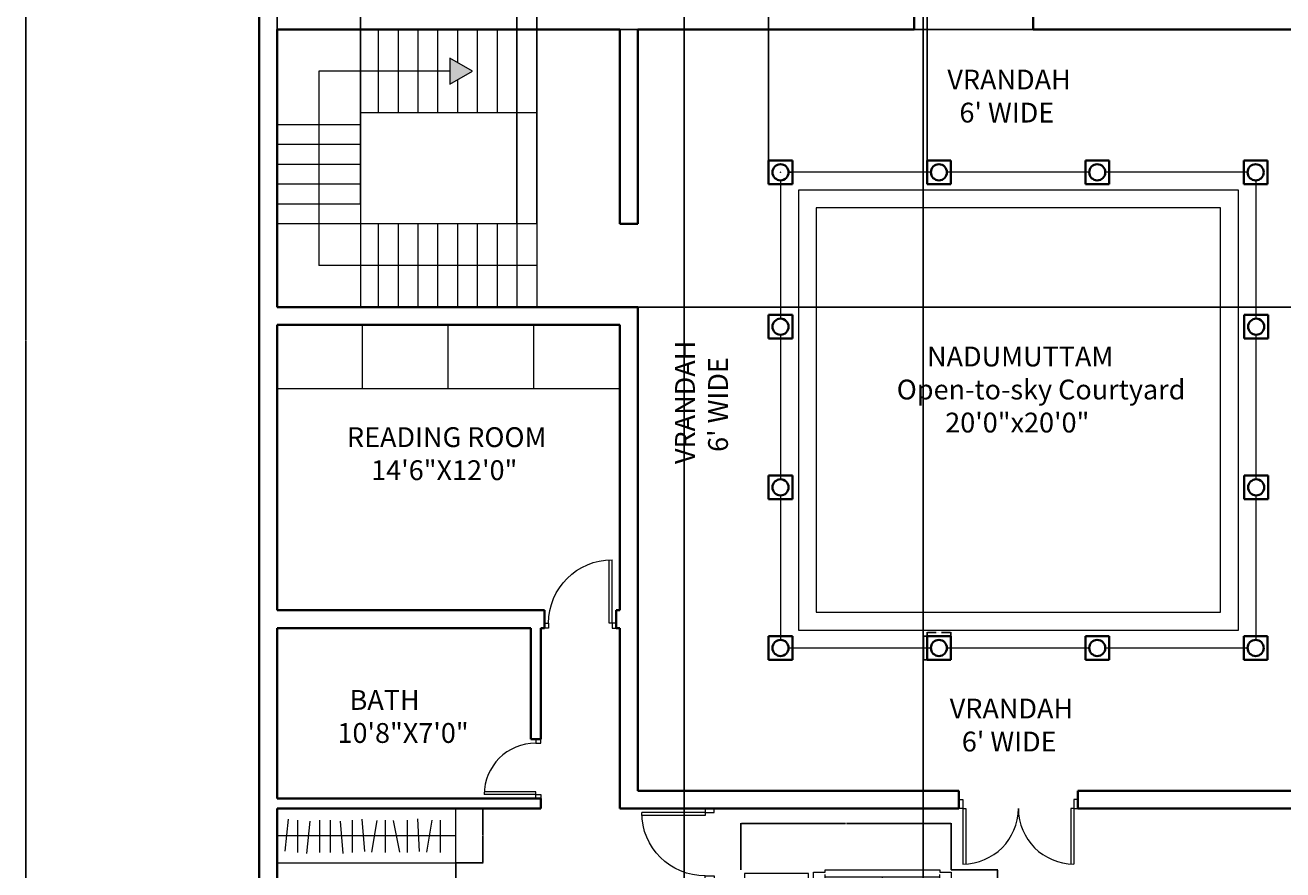
# Model space of a CAD drawing. Units: inches. Extents: x 4602 to 5612, y 5125 to 6591.
# Tile 2 of 6: x 4602 to 5237, y 5551 to 5977. Entities that reach past the tile are written whole.
import ezdxf

# ---------------------------------------------------------------- set-up
doc = ezdxf.new("R2010")
doc.units = ezdxf.units.IN
for name, color, linetype, lineweight in [('A-ANNO-DIMS', 2, 'Continuous', 18), ('A-ANNO-PATT', 7, 'Continuous', 18), ('A-ANNO-SYMB', 7, 'Continuous', 18), ('A-AREA-IDEN', 7, 'Continuous', 18), ('A-COLS', 7, 'Continuous', 35), ('A-DOOR', 4, 'Continuous', 18), ('A-FLOR-CASE', 9, 'Continuous', 18), ('A-FLOR-EDGE', 7, 'Continuous', 18), ('A-FLOR-STRS', 7, 'Continuous', 18), ('A-FURN', 8, 'Continuous', 13), ('A-WALL', 7, 'Continuous', 35)]:
    doc.layers.add(name, color=color, linetype=linetype, lineweight=lineweight)
doc.styles.get("Standard").update_dxf_attribs({"font": 'arial.ttf'})
doc.dimstyles.get("Standard").update_dxf_attribs({"dimtxt": 0.18, "dimasz": 0.18, "dimexe": 0.18, "dimexo": 0.0625, "dimgap": 0.09, "dimtad": 0, "dimtih": 1, "dimtoh": 1, "dimdec": 4, "dimzin": 0, "dimdsep": 46, "dimtxsty": 'Standard', "dimcen": 0.09, "dimadec": 0, "dimazin": 0, "dimtfac": 1, "dimtdec": 4, "dimtofl": 0, "dimtmove": 0, "dimatfit": 3, "dimfxl": 1, "dimtolj": 1, "dimtzin": 0, "dimarcsym": 0})

# ---------------------------------------------------------------- blocks, each defined once
blk = doc.blocks.new('A$C1C981678')
for p, q in [((0, 1425), (0, 2066)), ((0, 2066), (591, 2066)), ((55, 1480), (55, 2011)), ((55, 2011), (536, 2011)), ((536, 2011), (536, 1480)), ((591, 2066), (591, 1425)), ((643, 1571), (643, 2074)), ((643, 2074), (757, 2074)), ((757, 2097), (2312, 2097)), ((757, 2074), (757, 2097)), ((757, 1571), (757, 2074)), ((757, 2028), (2312, 2028)), ((1283, 1342), (1283, 2028)), ((1786, 1342), (1786, 2028)), ((2312, 2097), (2312, 2074)), ((2312, 2074), (2426, 2074)), ((2312, 1571), (2312, 2074)), ((2426, 2074), (2426, 1571)), ((2463, 2062), (2463, 1422)), ((3055, 2062), (2463, 2062)), ((3055, 1422), (3055, 2062)), ((2519, 2007), (2519, 1477)), ((3000, 2007), (2519, 2007)), ((3000, 1477), (3000, 2007)), ((287, 1770), (287, 1869)), ((2312, 1868), (757, 1868)), ((2312, 1822), (757, 1822)), ((2312, 1777), (757, 1777)), ((2773, 1759), (2773, 1859)), ((264, 1747), (165, 1747)), ((287, 1724), (287, 1625)), ((310, 1747), (409, 1747)), ((2750, 1737), (2651, 1737)), ((2773, 1714), (2773, 1615)), ((2796, 1737), (2895, 1737)), ((689, 1548), (643, 1571)), ((689, 1479), (689, 1548)), ((689, 1548), (734, 1548)), ((734, 1548), (757, 1571)), ((757, 1479), (757, 1571)), ((2335, 1548), (2312, 1571)), ((2312, 1479), (2312, 1571)), ((2380, 1548), (2335, 1548)), ((2426, 1571), (2380, 1548)), ((2380, 1548), (2380, 1479)), ((591, 1425), (0, 1425)), ((536, 1480), (55, 1480)), ((757, 1479), (689, 1479)), ((757, 1342), (757, 1479)), ((2380, 1479), (2312, 1479)), ((2312, 1479), (2312, 1342)), ((2463, 1422), (3055, 1422)), ((2519, 1477), (3000, 1477)), ((17, 1295), (17, 746)), ((40, 1295), (17, 1295)), ((634, 1364), (40, 1364)), ((40, 1364), (40, 1295)), ((108, 1295), (40, 1295)), ((345, 1295), (108, 1295)), ((108, 1295), (108, 746)), ((245, 746), (245, 1295)), ((295, 746), (295, 1295)), ((345, 746), (345, 1295)), ((345, 1295), (634, 1295)), ((634, 1295), (634, 1364)), ((680, 1295), (634, 1295)), ((680, 746), (680, 1295)), ((2312, 1342), (757, 1342)), ((2337, 114), (2337, 1257)), ((2337, 1257), (2475, 1257)), ((2475, 1326), (2543, 1326)), ((2475, 1257), (2475, 1326)), ((2475, 1257), (2566, 1257)), ((2543, 1326), (2566, 1372)), ((2543, 1326), (2543, 1280)), ((2543, 1280), (2566, 1257)), ((2566, 1372), (3069, 1372)), ((2566, 1257), (3046, 1257)), ((2772, 114), (2772, 1257)), ((2817, 114), (2817, 1257)), ((2863, 114), (2863, 1257)), ((3023, 1257), (3023, 114)), ((3069, 1372), (3069, 1257)), ((3069, 1257), (3092, 1257)), ((3092, 1257), (3092, 114)), ((1995, 1003), (1232, 1003)), ((1232, 1003), (1232, 659)), ((1960, 969), (1266, 969)), ((1266, 969), (1266, 694)), ((1960, 694), (1960, 969)), ((1995, 659), (1995, 1003)), ((17, 746), (40, 746)), ((40, 746), (40, 678)), ((108, 746), (40, 746)), ((40, 678), (634, 678)), ((108, 746), (345, 746)), ((634, 746), (345, 746)), ((634, 746), (680, 746)), ((634, 678), (634, 746)), ((1232, 659), (1995, 659)), ((1266, 694), (1960, 694)), ((2337, 686), (3023, 686)), ((2475, 114), (2337, 114)), ((2475, 46), (2475, 114)), ((2475, 114), (2566, 114)), ((2543, 46), (2475, 46)), ((2543, 91), (2566, 114)), ((2543, 46), (2543, 91)), ((2566, 0), (2543, 46)), ((2566, 114), (3046, 114)), ((3069, 0), (2566, 0)), ((3092, 114), (3069, 114)), ((3069, 114), (3069, 0))]:
    blk.add_line(p, q)
for radius in [122, 22.9]:
    blk.add_circle((2773, 1737), radius)
for major_axis in [(-86.2, 86.2), (16.2, 16.2)]:
    blk.add_ellipse((287, 1747), major_axis=major_axis, ratio=1)
blk = doc.blocks.new('DOOR-PAIR-60IN')
for p, q in [((2, 4.5), (2, 32.5)), ((3.5, 4.5), (3.5, 32.46)), ((56.5, 4.5), (56.5, 32.46)), ((58, 4.5), (58, 32.5)), ((2, 4.5), (0, 4.5)), ((2, 0), (2, 4.5)), ((2, 4.5), (3.5, 4.5)), ((58, 4.5), (56.5, 4.5)), ((58, 0), (58, 4.5)), ((58, 4.5), (60, 4.5)), ((0, 0), (2, 0)), ((60, 0), (58, 0))]:
    blk.add_line(p, q)
for centre, start, end in [((2, 4.5), 0, 90), ((58, 4.5), 90, 180)]:
    blk.add_arc(centre, 28, start, end)
blk = doc.blocks.new('DOOR-36IN-DEEP-JAMB')
for p, q in [((2, 4.5), (2, 36.5)), ((3.5, 4.5), (3.5, 36.46)), ((0, 4.5), (2, 4.5)), ((2, 4.5), (2, 0)), ((2, 4.5), (3.5, 4.5)), ((36, 4.5), (34, 4.5)), ((34, 4.5), (34, 0)), ((2, 0), (0, 0)), ((34, 0), (36, 0))]:
    blk.add_line(p, q)
blk.add_arc((2, 4.5), 32, 0, 90)
blk = doc.blocks.new('DOOR-36IN-SHALLOW-JAMB')
for p, q in [((2, 2.5), (2, 34.5)), ((3.5, 2.5), (3.5, 34.46)), ((0, 2.5), (2, 2.5)), ((2, 2.5), (2, 0)), ((2, 2.5), (3.5, 2.5)), ((36, 2.5), (34, 2.5)), ((34, 2.5), (34, 0)), ((2, 0), (0, 0)), ((34, 0), (36, 0))]:
    blk.add_line(p, q)
blk.add_arc((2, 2.5), 32, 0, 90)
blk = doc.blocks.new('DOOR-30IN')
for p, q in [((26, 30), (26, 28)), ((26, 28), (28.5, 28)), ((28.5, 28), (28.5, 30)), ((26, 2), (0, 2)), ((26, 3.5), (0.04, 3.5)), ((26, 2), (26, 3.5)), ((26, 0), (26, 2)), ((26, 2), (28.5, 2)), ((28.5, 2), (28.5, 0))]:
    blk.add_line(p, q)
blk.add_arc((26, 2), 26, 90, 180)
blk = doc.blocks.new('WARDROBE-RAIL')
for p, q in [((90.22, 0), (90.22, 27.46)), ((3.99, 5.88), (5.71, 22.16)), ((10.39, 5.25), (10.39, 21.62)), ((15.01, 4.71), (16.73, 21)), ((21.48, 5.25), (21.48, 21.62)), ((27.02, 5.25), (27.02, 21.62)), ((33.26, 4.83), (31.94, 21.15)), ((38.1, 5.25), (38.1, 21.62)), ((44.31, 5.72), (42.98, 22.05)), ((47.72, 5.36), (50.53, 21.49)), ((54.72, 5.25), (54.72, 21.62)), ((61.87, 5.4), (58.77, 21.48)), ((65.8, 5.25), (65.8, 21.62)), ((70.89, 22.2), (71.76, 5.85)), ((75.49, 5.36), (78.19, 21.52)), ((82.43, 5.25), (82.43, 21.62)), ((90.22, 13.73), (0, 13.73)), ((0, 0), (90.22, 0))]:
    blk.add_line(p, q)
blk = doc.blocks.new('POST-NADUMUTTAM')
for p, q in [((12, 12), (0, 12)), ((0, 12), (0, 0)), ((12, 0), (12, 12)), ((12, 0), (0, 0))]:
    blk.add_line(p, q)
blk.add_circle((6, 6), 4.06)
blk = doc.blocks.new('*D19')
at = {"layer": 'A-ANNO-DIMS', "color": 0, "lineweight": -2, "transparency": 16777216}
for p, q in [((5057.15, 5668.61), (5057.15, 5670.53)), ((5057.33, 5670.35), (5061.76, 5670.35)), ((5068.97, 5670.35), (5064.54, 5670.35)), ((5069.15, 5668.61), (5069.15, 5670.53))]:
    blk.add_line(p, q, dxfattribs=at)
at = {"layer": 'A-ANNO-DIMS', "color": 0, "transparency": 16777216}
for points in [[(5057.33, 5670.38), (5057.33, 5670.32), (5057.15, 5670.35)], [(5068.97, 5670.38), (5068.97, 5670.32), (5069.15, 5670.35)]]:
    blk.add_solid(points, dxfattribs=at)
at = {"layer": 'Defpoints', "color": 0, "transparency": 16777216}
for p in [(5057.15, 5668.55), (5069.15, 5670.35), (5069.15, 5668.55)]:
    blk.add_point(p, dxfattribs=at)
at = {"layer": 'A-ANNO-DIMS', "color": 0, "transparency": 16777216, "insert": (5063.15, 5670.35), "char_height": 0.18, "attachment_point": 5}
blk.add_mtext('\\A1;COURT POST 12 TYP.', dxfattribs=at)
blk = doc.blocks.new('*D20')
at = {"layer": 'A-ANNO-DIMS', "color": 0, "lineweight": -2, "transparency": 16777216}
for p, q in [((5057.09, 5668.55), (5055.17, 5668.55)), ((5055.35, 5668.37), (5055.35, 5662.73)), ((5055.35, 5656.73), (5055.35, 5662.37)), ((5057.09, 5656.55), (5055.17, 5656.55))]:
    blk.add_line(p, q, dxfattribs=at)
at = {"layer": 'A-ANNO-DIMS', "color": 0, "transparency": 16777216}
for points in [[(5055.32, 5668.37), (5055.38, 5668.37), (5055.35, 5668.55)], [(5055.32, 5656.73), (5055.38, 5656.73), (5055.35, 5656.55)]]:
    blk.add_solid(points, dxfattribs=at)
at = {"layer": 'Defpoints', "color": 0, "transparency": 16777216}
for p in [(5055.35, 5668.55), (5057.15, 5668.55), (5057.15, 5656.55)]:
    blk.add_point(p, dxfattribs=at)
at = {"layer": 'A-ANNO-DIMS', "color": 0, "transparency": 16777216, "insert": (5055.35, 5662.55), "char_height": 0.18, "attachment_point": 5}
blk.add_mtext('\\A1;12 TYP.', dxfattribs=at)
blk = doc.blocks.new('*D39')
at = {"layer": 'A-ANNO-DIMS', "color": 0, "lineweight": -2, "transparency": 16777216}
for p, q in [((4729.24, 5554.03), (4729.24, 5540.38)), ((4819.46, 5554.03), (4819.46, 5540.38)), ((4729.42, 5540.56), (4773.04, 5540.56)), ((4819.28, 5540.56), (4775.66, 5540.56))]:
    blk.add_line(p, q, dxfattribs=at)
at = {"layer": 'A-ANNO-DIMS', "color": 0, "transparency": 16777216}
for points in [[(4729.42, 5540.59), (4729.42, 5540.53), (4729.24, 5540.56)], [(4819.28, 5540.59), (4819.28, 5540.53), (4819.46, 5540.56)]]:
    blk.add_solid(points, dxfattribs=at)
at = {"layer": 'Defpoints', "color": 0, "transparency": 16777216}
for p in [(4729.24, 5554.09), (4819.46, 5554.09), (4819.46, 5540.56)]:
    blk.add_point(p, dxfattribs=at)
at = {"layer": 'A-ANNO-DIMS', "color": 0, "transparency": 16777216, "insert": (4774.35, 5540.56), "char_height": 0.18, "attachment_point": 5}
blk.add_mtext('\\A1;WARDROBE 90 TYP.', dxfattribs=at)
blk = doc.blocks.new('*D40')
at = {"layer": 'A-ANNO-DIMS', "color": 0, "lineweight": -2, "transparency": 16777216}
for p, q in [((4819.52, 5581.55), (4833.17, 5581.55)), ((4832.99, 5581.37), (4832.99, 5568)), ((4832.99, 5554.27), (4832.99, 5567.64)), ((4819.52, 5554.09), (4833.17, 5554.09))]:
    blk.add_line(p, q, dxfattribs=at)
at = {"layer": 'A-ANNO-DIMS', "color": 0, "transparency": 16777216}
for points in [[(4832.96, 5581.37), (4833.02, 5581.37), (4832.99, 5581.55)], [(4832.96, 5554.27), (4833.02, 5554.27), (4832.99, 5554.09)]]:
    blk.add_solid(points, dxfattribs=at)
at = {"layer": 'Defpoints', "color": 0, "transparency": 16777216}
for p in [(4819.46, 5581.55), (4832.99, 5581.55), (4819.46, 5554.09)]:
    blk.add_point(p, dxfattribs=at)
at = {"layer": 'A-ANNO-DIMS', "color": 0, "transparency": 16777216, "insert": (4832.99, 5567.82), "char_height": 0.18, "attachment_point": 5}
blk.add_mtext('\\A1;27 TYP.', dxfattribs=at)
blk = doc.blocks.new('*D51')
at = {"layer": 'A-ANNO-DIMS', "color": 0, "lineweight": -2, "transparency": 16777216}
for p, q in [((5069.38, 5550.61), (5092.95, 5550.61)), ((5092.77, 5550.43), (5092.77, 5472.63)), ((5092.77, 5394.45), (5092.77, 5472.26)), ((5069.38, 5394.27), (5092.95, 5394.27))]:
    blk.add_line(p, q, dxfattribs=at)
at = {"layer": 'A-ANNO-DIMS', "color": 0, "transparency": 16777216}
for points in [[(5092.74, 5550.43), (5092.8, 5550.43), (5092.77, 5550.61)], [(5092.74, 5394.45), (5092.8, 5394.45), (5092.77, 5394.27)]]:
    blk.add_solid(points, dxfattribs=at)
at = {"layer": 'Defpoints', "color": 0, "transparency": 16777216}
for p in [(5069.32, 5550.61), (5092.77, 5550.61), (5069.32, 5394.27)]:
    blk.add_point(p, dxfattribs=at)
at = {"layer": 'A-ANNO-DIMS', "color": 0, "transparency": 16777216, "insert": (5092.77, 5472.44), "char_height": 0.18, "attachment_point": 5}
blk.add_mtext('\\A1;LIVING SEATING 156', dxfattribs=at)
blk = doc.blocks.new('*D52')
at = {"layer": 'A-ANNO-DIMS', "color": 0, "lineweight": -2, "transparency": 16777216}
for p, q in [((4963.3, 5550.68), (4963.3, 5574.25)), ((4963.48, 5574.07), (5016.03, 5574.07)), ((5069.14, 5574.07), (5016.59, 5574.07)), ((5069.32, 5550.68), (5069.32, 5574.25))]:
    blk.add_line(p, q, dxfattribs=at)
at = {"layer": 'A-ANNO-DIMS', "color": 0, "transparency": 16777216}
for points in [[(4963.48, 5574.1), (4963.48, 5574.04), (4963.3, 5574.07)], [(5069.14, 5574.1), (5069.14, 5574.04), (5069.32, 5574.07)]]:
    blk.add_solid(points, dxfattribs=at)
at = {"layer": 'Defpoints', "color": 0, "transparency": 16777216}
for p in [(4963.3, 5574.07), (4963.3, 5550.61), (5069.32, 5550.61)]:
    blk.add_point(p, dxfattribs=at)
at = {"layer": 'A-ANNO-DIMS', "color": 0, "transparency": 16777216, "insert": (5016.31, 5574.07), "char_height": 0.18, "attachment_point": 5}
blk.add_mtext('\\A1;106', dxfattribs=at)
blk = doc.blocks.new('*D56')
at = {"layer": 'A-ANNO-DIMS', "color": 0, "lineweight": -2, "transparency": 16777216}
for p, q in [((5061.18, 6438.55), (4602.21, 6438.55)), ((4602.39, 6438.37), (4602.39, 5817.73)), ((4602.39, 5196.73), (4602.39, 5817.37)), ((5055.18, 5196.55), (4602.21, 5196.55))]:
    blk.add_line(p, q, dxfattribs=at)
at = {"layer": 'A-ANNO-DIMS', "color": 0, "transparency": 16777216}
for points in [[(4602.36, 6438.37), (4602.42, 6438.37), (4602.39, 6438.55)], [(4602.36, 5196.73), (4602.42, 5196.73), (4602.39, 5196.55)]]:
    blk.add_solid(points, dxfattribs=at)
at = {"layer": 'Defpoints', "color": 0, "transparency": 16777216}
for p in [(4602.39, 6438.55), (5061.24, 6438.55), (5055.24, 5196.55)]:
    blk.add_point(p, dxfattribs=at)
at = {"layer": 'A-ANNO-DIMS', "color": 0, "transparency": 16777216, "insert": (4602.39, 5817.55), "char_height": 0.18, "attachment_point": 5}
blk.add_mtext('\\A1;1242', dxfattribs=at)
blk = doc.blocks.new('*D59')
at = {"layer": 'A-ANNO-DIMS', "color": 0, "lineweight": -2, "transparency": 16777216}
for p, q in [((4977.24, 5908.61), (4977.24, 6572.85)), ((4977.42, 6572.67), (5016.82, 6572.67)), ((5056.97, 6572.67), (5017.57, 6572.67)), ((5057.15, 5908.61), (5057.15, 6572.85))]:
    blk.add_line(p, q, dxfattribs=at)
at = {"layer": 'A-ANNO-DIMS', "color": 0, "transparency": 16777216}
for points in [[(4977.42, 6572.7), (4977.42, 6572.64), (4977.24, 6572.67)], [(5056.97, 6572.7), (5056.97, 6572.64), (5057.15, 6572.67)]]:
    blk.add_solid(points, dxfattribs=at)
at = {"layer": 'Defpoints', "color": 0, "transparency": 16777216}
for p in [(5057.15, 6572.67), (4977.24, 5908.55), (5057.15, 5908.55)]:
    blk.add_point(p, dxfattribs=at)
at = {"layer": 'A-ANNO-DIMS', "color": 0, "transparency": 16777216, "insert": (5017.19, 6572.67), "char_height": 0.18, "attachment_point": 5}
blk.add_mtext('\\A1;79.91', dxfattribs=at)
blk = doc.blocks.new('*D60')
at = {"layer": 'A-ANNO-DIMS', "color": 0, "lineweight": -2, "transparency": 16777216}
for p, q in [((4934.59, 5248.61), (4934.59, 6572.85)), ((4934.77, 6572.67), (4994.46, 6572.67)), ((5055.06, 6572.67), (4995.37, 6572.67)), ((5055.24, 5248.61), (5055.24, 6572.85))]:
    blk.add_line(p, q, dxfattribs=at)
at = {"layer": 'A-ANNO-DIMS', "color": 0, "transparency": 16777216}
for points in [[(4934.77, 6572.7), (4934.77, 6572.64), (4934.59, 6572.67)], [(5055.06, 6572.7), (5055.06, 6572.64), (5055.24, 6572.67)]]:
    blk.add_solid(points, dxfattribs=at)
at = {"layer": 'Defpoints', "color": 0, "transparency": 16777216}
for p in [(5055.24, 6572.67), (4934.59, 5248.55), (5055.24, 5248.55)]:
    blk.add_point(p, dxfattribs=at)
at = {"layer": 'A-ANNO-DIMS', "color": 0, "transparency": 16777216, "insert": (4994.91, 6572.67), "char_height": 0.18, "attachment_point": 5}
blk.add_mtext('\\A1;120.65', dxfattribs=at)
blk = doc.blocks.new('*D62')
at = {"layer": 'A-ANNO-DIMS', "color": 0, "lineweight": -2, "transparency": 16777216}
for p, q in [((4729.24, 5886.61), (4729.24, 6572.85)), ((4729.42, 6572.67), (4750.02, 6572.67)), ((4771.06, 6572.67), (4750.46, 6572.67)), ((4771.24, 5886.61), (4771.24, 6572.85))]:
    blk.add_line(p, q, dxfattribs=at)
at = {"layer": 'A-ANNO-DIMS', "color": 0, "transparency": 16777216}
for points in [[(4729.42, 6572.7), (4729.42, 6572.64), (4729.24, 6572.67)], [(4771.06, 6572.7), (4771.06, 6572.64), (4771.24, 6572.67)]]:
    blk.add_solid(points, dxfattribs=at)
at = {"layer": 'Defpoints', "color": 0, "transparency": 16777216}
for p in [(4771.24, 6572.67), (4729.24, 5886.55), (4771.24, 5886.55)]:
    blk.add_point(p, dxfattribs=at)
at = {"layer": 'A-ANNO-DIMS', "color": 0, "transparency": 16777216, "insert": (4750.24, 6572.67), "char_height": 0.18, "attachment_point": 5}
blk.add_mtext('\\A1;42', dxfattribs=at)
blk = doc.blocks.new('*D63')
at = {"layer": 'A-ANNO-DIMS', "color": 0, "lineweight": -2, "transparency": 16777216}
for p, q in [((4850.24, 5876.61), (4850.24, 6572.85)), ((4850.42, 6572.67), (4855.03, 6572.67)), ((4860.06, 6572.67), (4855.45, 6572.67)), ((4860.24, 5876.61), (4860.24, 6572.85))]:
    blk.add_line(p, q, dxfattribs=at)
at = {"layer": 'A-ANNO-DIMS', "color": 0, "transparency": 16777216}
for points in [[(4850.42, 6572.7), (4850.42, 6572.64), (4850.24, 6572.67)], [(4860.06, 6572.7), (4860.06, 6572.64), (4860.24, 6572.67)]]:
    blk.add_solid(points, dxfattribs=at)
at = {"layer": 'Defpoints', "color": 0, "transparency": 16777216}
for p in [(4860.24, 6572.67), (4850.24, 5876.55), (4860.24, 5876.55)]:
    blk.add_point(p, dxfattribs=at)
at = {"layer": 'A-ANNO-DIMS', "color": 0, "transparency": 16777216, "insert": (4855.24, 6572.67), "char_height": 0.18, "attachment_point": 5}
blk.add_mtext('\\A1;10', dxfattribs=at)
blk = doc.blocks.new('*D64')
at = {"layer": 'A-ANNO-DIMS', "color": 0, "lineweight": -2, "transparency": 16777216}
for p, q in [((4860.3, 5974.55), (5612.27, 5974.55)), ((5612.09, 5974.37), (5612.09, 5904.73)), ((5612.09, 5834.73), (5612.09, 5904.37)), ((4860.3, 5834.55), (5612.27, 5834.55))]:
    blk.add_line(p, q, dxfattribs=at)
at = {"layer": 'A-ANNO-DIMS', "color": 0, "transparency": 16777216}
for points in [[(5612.06, 5974.37), (5612.12, 5974.37), (5612.09, 5974.55)], [(5612.06, 5834.73), (5612.12, 5834.73), (5612.09, 5834.55)]]:
    blk.add_solid(points, dxfattribs=at)
at = {"layer": 'Defpoints', "color": 0, "transparency": 16777216}
for p in [(4860.24, 5974.55), (5612.09, 5974.55), (4860.24, 5834.55)]:
    blk.add_point(p, dxfattribs=at)
at = {"layer": 'A-ANNO-DIMS', "color": 0, "transparency": 16777216, "insert": (5612.09, 5904.55), "char_height": 0.18, "attachment_point": 5}
blk.add_mtext('\\A1;140', dxfattribs=at)
blk = doc.blocks.new('*D72')
at = {"layer": 'A-ANNO-DIMS', "color": 0, "lineweight": -2, "transparency": 16777216}
for p, q in [((4983.15, 5902.55), (4983.33, 5902.55)), ((4983.24, 5902.46), (4983.24, 5902.64)), ((4989.73, 5902.55), (4987.48, 5902.55))]:
    blk.add_line(p, q, dxfattribs=at)
at = {"layer": 'A-ANNO-DIMS', "color": 0, "transparency": 16777216}
blk.add_solid([(4987.48, 5902.58), (4987.48, 5902.52), (4987.3, 5902.55)], dxfattribs=at)
at = {"layer": 'Defpoints', "color": 0, "transparency": 16777216}
for p in [(4979.18, 5902.55), (4987.3, 5902.55)]:
    blk.add_point(p, dxfattribs=at)
at = {"layer": 'A-ANNO-DIMS', "color": 0, "transparency": 16777216, "insert": (4990.48, 5902.55), "char_height": 0.18, "attachment_point": 5}
blk.add_mtext('\\A1;12X ∅8.118', dxfattribs=at)

msp = doc.modelspace()

# ---------------------------------------------------------------- hatches: boundary and pattern name
at = {"layer": 'A-ANNO-PATT'}
h = msp.add_hatch(color=256, dxfattribs=at)
h.dxf.hatch_style = 1
h.paths.add_polyline_path([(4827.7715, 5953.5515), (4816.4728, 5960.0748), (4816.4728, 5947.0283)])

# ---------------------------------------------------------------- linework, layer by layer
at = {"layer": 'A-ANNO-SYMB'}
for p, q in [((4750.239, 5953.5515), (4750.239, 5855.5515)), ((4816.4728, 5953.5515), (4750.239, 5953.5515)), ((4860.239, 5855.5515), (4750.239, 5855.5515))]:
    msp.add_line(p, q, dxfattribs=at)
msp.add_lwpolyline([(4827.7715, 5953.5515), (4816.4728, 5960.0748), (4816.4728, 5947.0283)], close=True, dxfattribs=at)
at = {"layer": 'A-FLOR-CASE'}
for p, q in [((4772.4066, 5793.4433), (4772.4066, 5825.5515)), ((4815.5741, 5793.4433), (4815.5741, 5825.5515)), ((4858.7417, 5793.4433), (4858.7417, 5825.5515)), ((4729.239, 5793.4433), (4902.239, 5793.4433))]:
    msp.add_line(p, q, dxfattribs=at)
at = {"layer": 'A-FLOR-EDGE'}
for points in [[(5059.0906, 5902.5515), (4987.2981, 5902.5515)], [(5139.0013, 5902.5515), (5067.2087, 5902.5515)], [(5218.9119, 5902.5515), (5147.1194, 5902.5515)], [(4983.239, 5898.4925), (4983.239, 5828.7154)], [(5223.239, 5828.7154), (5223.239, 5898.5013)], [(4983.239, 5820.5972), (4983.239, 5747.663)], [(5223.239, 5747.663), (5223.239, 5820.5972)], [(4983.239, 5739.5449), (4983.239, 5666.6106)], [(5223.239, 5666.6017), (5223.239, 5739.5449)], [(4987.2981, 5662.5515), (5059.0906, 5662.5515)], [(5067.2087, 5662.5515), (5139.0013, 5662.5515)], [(5147.1194, 5662.5515), (5218.9119, 5662.5515)]]:
    msp.add_lwpolyline(points, dxfattribs=at)
for points in [[(4992.239, 5893.5515), (4992.239, 5671.5515), (5214.239, 5671.5515), (5214.239, 5893.5515)], [(5001.239, 5884.5515), (5001.239, 5680.5515), (5205.239, 5680.5515), (5205.239, 5884.5515)]]:
    msp.add_lwpolyline(points, close=True, dxfattribs=at)
at = {"layer": 'A-FLOR-STRS'}
for p, q in [((4771.239, 5974.5515), (4771.239, 5834.5515)), ((4780.239, 5974.5515), (4780.239, 5932.5515)), ((4790.239, 5974.5515), (4790.239, 5932.5515)), ((4800.239, 5974.5515), (4800.239, 5932.5515)), ((4810.239, 5974.5515), (4810.239, 5932.5515)), ((4820.239, 5974.5515), (4820.239, 5957.9004)), ((4830.239, 5974.5515), (4830.239, 5932.5515)), ((4840.239, 5974.5515), (4840.239, 5932.5515)), ((4850.239, 5974.5515), (4850.239, 5932.5515)), ((4860.239, 5974.5515), (4860.239, 5932.5515)), ((4820.239, 5949.2027), (4820.239, 5932.5515)), ((4860.239, 5932.5515), (4771.239, 5932.5515)), ((4771.239, 5926.5515), (4729.239, 5926.5515)), ((4771.239, 5916.5515), (4729.239, 5916.5515)), ((4771.239, 5906.5515), (4729.239, 5906.5515)), ((4771.239, 5896.5515), (4729.239, 5896.5515)), ((4771.239, 5886.5515), (4729.239, 5886.5515)), ((4860.239, 5876.5515), (4729.239, 5876.5515)), ((4780.239, 5876.5515), (4780.239, 5834.5515)), ((4790.239, 5876.5515), (4790.239, 5834.5515)), ((4800.239, 5876.5515), (4800.239, 5834.5515)), ((4810.239, 5876.5515), (4810.239, 5834.5515)), ((4820.239, 5876.5515), (4820.239, 5834.5515)), ((4830.239, 5876.5515), (4830.239, 5834.5515)), ((4840.239, 5876.5515), (4840.239, 5834.5515)), ((4850.239, 5876.5515), (4850.239, 5834.5515)), ((4860.239, 5876.5515), (4860.239, 5834.5515))]:
    msp.add_line(p, q, dxfattribs=at)
at = {"layer": 'A-WALL'}
for p, q in [((4720.239, 6208.5515), (4720.239, 5380.5515)), ((5050.739, 5983.5515), (5050.739, 5974.5515)), ((5110.739, 5983.5515), (5110.739, 5974.5515)), ((4729.239, 5974.5515), (4729.239, 5834.5515)), ((4902.239, 5974.5515), (4729.239, 5974.5515)), ((4902.239, 5974.5515), (4902.239, 5876.5515)), ((4911.239, 5974.5515), (4911.239, 5876.5515)), ((5050.739, 5974.5515), (4911.239, 5974.5515)), ((5295.239, 5974.5515), (5110.739, 5974.5515)), ((4911.239, 5876.5515), (4902.239, 5876.5515)), ((4911.239, 5834.5515), (4729.239, 5834.5515)), ((4911.239, 5834.5515), (4911.239, 5590.5515)), ((4902.239, 5825.5515), (4729.239, 5825.5515)), ((4729.239, 5825.5515), (4729.239, 5681.5515)), ((4902.239, 5825.5515), (4902.239, 5681.5515)), ((4862.239, 5681.5515), (4729.239, 5681.5515)), ((4862.239, 5681.5515), (4864.239, 5681.5515)), ((4864.239, 5681.5515), (4864.239, 5672.5515)), ((4900.239, 5672.5515), (4900.239, 5681.5515)), ((4900.239, 5681.5515), (4902.239, 5681.5515)), ((4857.239, 5672.5515), (4729.239, 5672.5515)), ((4729.239, 5672.5515), (4729.239, 5586.5515)), ((4857.239, 5672.5515), (4857.239, 5616.5515)), ((4862.239, 5672.5515), (4862.239, 5616.5515)), ((4864.239, 5672.5515), (4862.239, 5672.5515)), ((4900.239, 5672.5515), (4902.239, 5672.5515)), ((4902.239, 5672.5515), (4902.239, 5581.5515)), ((4862.239, 5616.5515), (4857.239, 5616.5515)), ((4862.239, 5586.5515), (4729.239, 5586.5515)), ((4862.239, 5586.5515), (4862.239, 5581.5515)), ((5073.239, 5590.5515), (4911.239, 5590.5515)), ((5073.239, 5590.5515), (5073.239, 5581.5515)), ((5295.239, 5590.5515), (5133.239, 5590.5515)), ((5133.239, 5590.5515), (5133.239, 5581.5515)), ((4862.239, 5581.5515), (4729.239, 5581.5515)), ((4729.239, 5581.5515), (4729.239, 5389.5515)), ((5073.239, 5581.5515), (4902.239, 5581.5515)), ((5304.239, 5581.5515), (5133.239, 5581.5515))]:
    msp.add_line(p, q, dxfattribs=at)

# ---------------------------------------------------------------- block references
at = {"layer": 'A-COLS'}
for p in [(4977.239, 5896.552), (5057.1496, 5896.552), (5137.0603, 5896.552), (5216.9709, 5896.552), (4977.239, 5818.6568), (5217.239, 5818.6568), (4977.239, 5737.6044), (5217.239, 5737.6044), (4977.239, 5656.552), (5057.1496, 5656.552), (5137.0603, 5656.552), (5216.9709, 5656.552)]:
    msp.add_blockref('POST-NADUMUTTAM', p, dxfattribs=at)
at = {"layer": 'A-DOOR', "extrusion": (0, 0, -1), "zscale": -1}
msp.add_blockref('DOOR-36IN-SHALLOW-JAMB', (-4900.2391, 5672.552), dxfattribs=at)
at = {"layer": 'A-DOOR'}
msp.add_blockref('DOOR-30IN', (4833.739, 5586.552), dxfattribs=at)
at = {"layer": 'A-DOOR', "rotation": 180}
msp.add_blockref('DOOR-PAIR-60IN', (5133.2391, 5586.051), dxfattribs=at)
at = {"layer": 'A-DOOR', "extrusion": (0, 0, -1), "zscale": -1, "rotation": 270.0000000000028}
msp.add_blockref('DOOR-36IN-DEEP-JAMB', (-4949.7386, 5581.5516), dxfattribs=at)
at = {"layer": 'A-FLOR-CASE'}
msp.add_blockref('WARDROBE-RAIL', (4729.239, 5554.094), dxfattribs=at)
at = {"layer": 'A-FURN', "xscale": 0.0505668113949487, "yscale": 0.0505668113949487, "zscale": 0.0505668113949487, "rotation": 90}
msp.add_blockref('A$C1C981678', (5069.3208, 5394.2739), dxfattribs=at)

# ---------------------------------------------------------------- texts
at = {"layer": 'A-AREA-IDEN', "char_height": 10, "attachment_point": 1}
for s, width, insert in [("VRANDAH\\P  6' WIDE", 127.373556, (5067.4101, 5954.3416)), ('     NADUMUTTAM\\POpen-to-sky Courtyard\\P        20\'0"x20\'0"', 231.362216, (5041.8896, 5814.6233)), ('READING ROOM\\P    14\'6"X12\'0"', 140.595401, (4764.4765, 5773.9224)), ('  BATH \\P10\'8"X7\'0"', 127.373556, (4759.6949, 5641.3427)), ("VRANDAH\\P  6' WIDE", 127.373556, (5068.6082, 5636.9991))]:
    msp.add_mtext_dynamic_manual_height_columns(s, width=width, gutter_width=12.5, heights=[0], dxfattribs=dict(at, insert=insert))
at = {"layer": 'A-AREA-IDEN', "insert": (4930.0425, 5755.357), "char_height": 10, "attachment_point": 1, "rotation": 90}
msp.add_mtext_dynamic_manual_height_columns("VRANDAH\\P  6' WIDE", width=127.373556, gutter_width=12.5, heights=[0], dxfattribs=at)

# ---------------------------------------------------------------- dimensions: what is measured, and where the dimension line sits
at = {"layer": 'A-ANNO-DIMS'}
for base, p1, p2, override, picture, middle in [((4771.239, 6572.6716), (4729.239, 5886.5515), (4771.239, 5886.5515), {"dimdec": 0, "dimlfac": 1, "dimrnd": 0, "dimzin": 0, "dimdsep": 46, "dimlunit": 2}, '*D62', (4750.239, 6572.6716)), ((4860.239, 6572.6716), (4850.239, 5876.5515), (4860.239, 5876.5515), {"dimdec": 0, "dimlfac": 1, "dimrnd": 0, "dimzin": 0, "dimdsep": 46, "dimlunit": 2}, '*D63', (4855.239, 6572.6716)), ((5055.239, 6572.6716), (4934.5878, 5248.5515), (5055.239, 5248.5515), {"dimdec": 2, "dimlfac": 1, "dimrnd": 0, "dimzin": 0, "dimdsep": 46, "dimlunit": 2}, '*D60', (4994.9134, 6572.6716)), ((5057.1497, 6572.6716), (4977.239, 5908.5515), (5057.1497, 5908.5515), {"dimdec": 2, "dimlfac": 1, "dimrnd": 0, "dimzin": 0, "dimdsep": 46, "dimlunit": 2}, '*D59', (5017.1944, 6572.6716))]:
    dim = msp.add_linear_dim(base=base, p1=p1, p2=p2, dimstyle='Standard', override=override, dxfattribs=at)
    dim.commit()
    dim.dimension.update_dxf_attribs({"geometry": picture, "text_midpoint": middle})
for base, p1, p2, angle, picture, middle in [((4602.389, 6438.5515), (5055.239, 5196.5515), (5061.239, 6438.5515), 90, '*D56', (4602.389, 5817.5515)), ((5612.089, 5974.5515), (4860.239, 5834.5515), (4860.239, 5974.5515), 90, '*D64', (5612.089, 5904.5515)), ((4963.2986, 5574.0654), (5069.3208, 5550.6143), (4963.2986, 5550.6143), 180, '*D52', (5016.3097, 5574.0654))]:
    dim = msp.add_linear_dim(base=base, p1=p1, p2=p2, angle=angle, dimstyle='Standard', override={"dimdec": 0, "dimlfac": 1, "dimrnd": 0, "dimzin": 0, "dimdsep": 46, "dimlunit": 2}, dxfattribs=at)
    dim.commit()
    dim.dimension.update_dxf_attribs({"geometry": picture, "text_midpoint": middle})
dim = msp.add_diameter_dim_2p(p1=(4979.18, 5902.5531), p2=(4987.2981, 5902.55), text='12X <>', dimstyle='Standard', override={"dimdec": 3, "dimlfac": 1, "dimrnd": 0, "dimzin": 0, "dimdsep": 46, "dimlunit": 2}, dxfattribs=at)
dim.commit()
dim.dimension.update_dxf_attribs({"geometry": '*D72', "text_midpoint": (4989.7335, 5902.5491), "dimtype": 163})
for base, p1, p2, text, picture, middle in [((5055.3497, 5668.5515), (5057.1497, 5656.5515), (5057.1497, 5668.5515), '<> TYP.', '*D20', (5055.3497, 5662.5515)), ((4832.9947, 5581.5515), (4819.4613, 5554.0942), (4819.4613, 5581.5515), '<> TYP.', '*D40', (4832.9947, 5567.8229)), ((5092.7719, 5550.6143), (5069.3208, 5394.2739), (5069.3208, 5550.6143), 'LIVING SEATING <>', '*D51', (5092.7719, 5472.4441))]:
    dim = msp.add_linear_dim(base=base, p1=p1, p2=p2, angle=90, text=text, dimstyle='Standard', override={"dimdec": 0, "dimlfac": 1, "dimrnd": 0, "dimzin": 0, "dimdsep": 46, "dimlunit": 2}, dxfattribs=at)
    dim.commit()
    dim.dimension.update_dxf_attribs({"geometry": picture, "text_midpoint": middle})
for base, p1, p2, text, picture, middle in [((5069.1497, 5670.3515), (5057.1497, 5668.5515), (5069.1497, 5668.5515), 'COURT POST <> TYP.', '*D19', (5063.1497, 5670.3515)), ((4819.4613, 5540.5608), (4729.239, 5554.0942), (4819.4613, 5554.0942), 'WARDROBE <> TYP.', '*D39', (4774.3502, 5540.5608))]:
    dim = msp.add_linear_dim(base=base, p1=p1, p2=p2, text=text, dimstyle='Standard', override={"dimdec": 0, "dimlfac": 1, "dimrnd": 0, "dimzin": 0, "dimdsep": 46, "dimlunit": 2}, dxfattribs=at)
    dim.commit()
    dim.dimension.update_dxf_attribs({"geometry": picture, "text_midpoint": middle})

doc.saveas('drawing.dxf')
